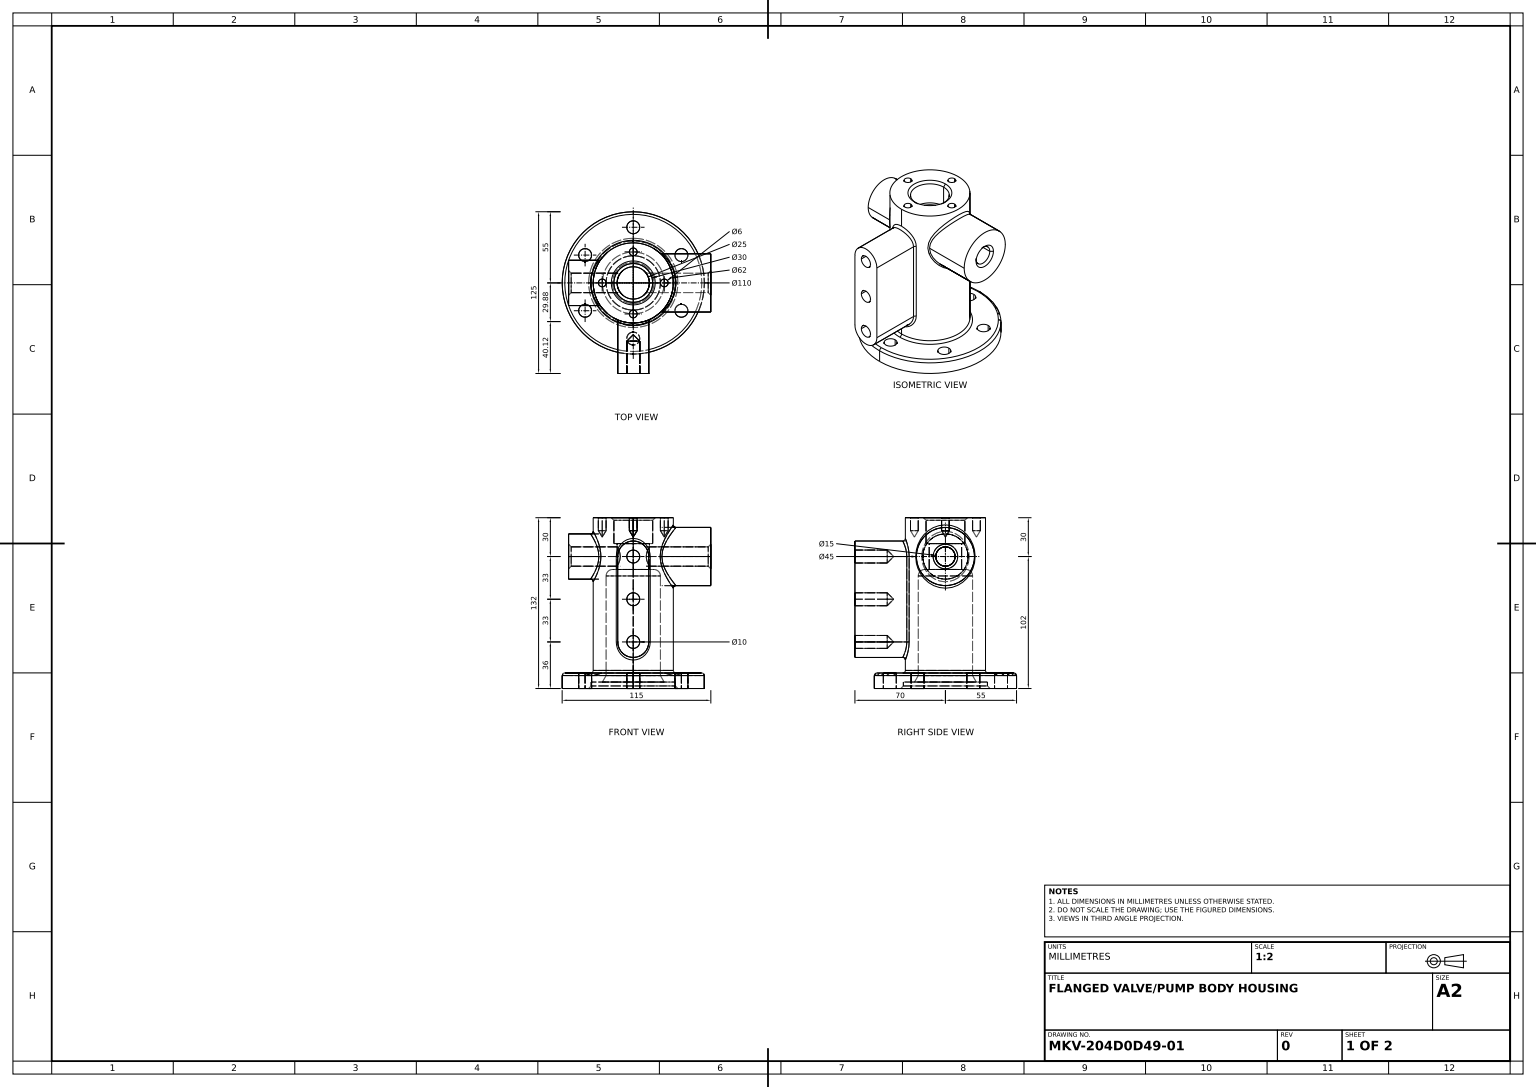
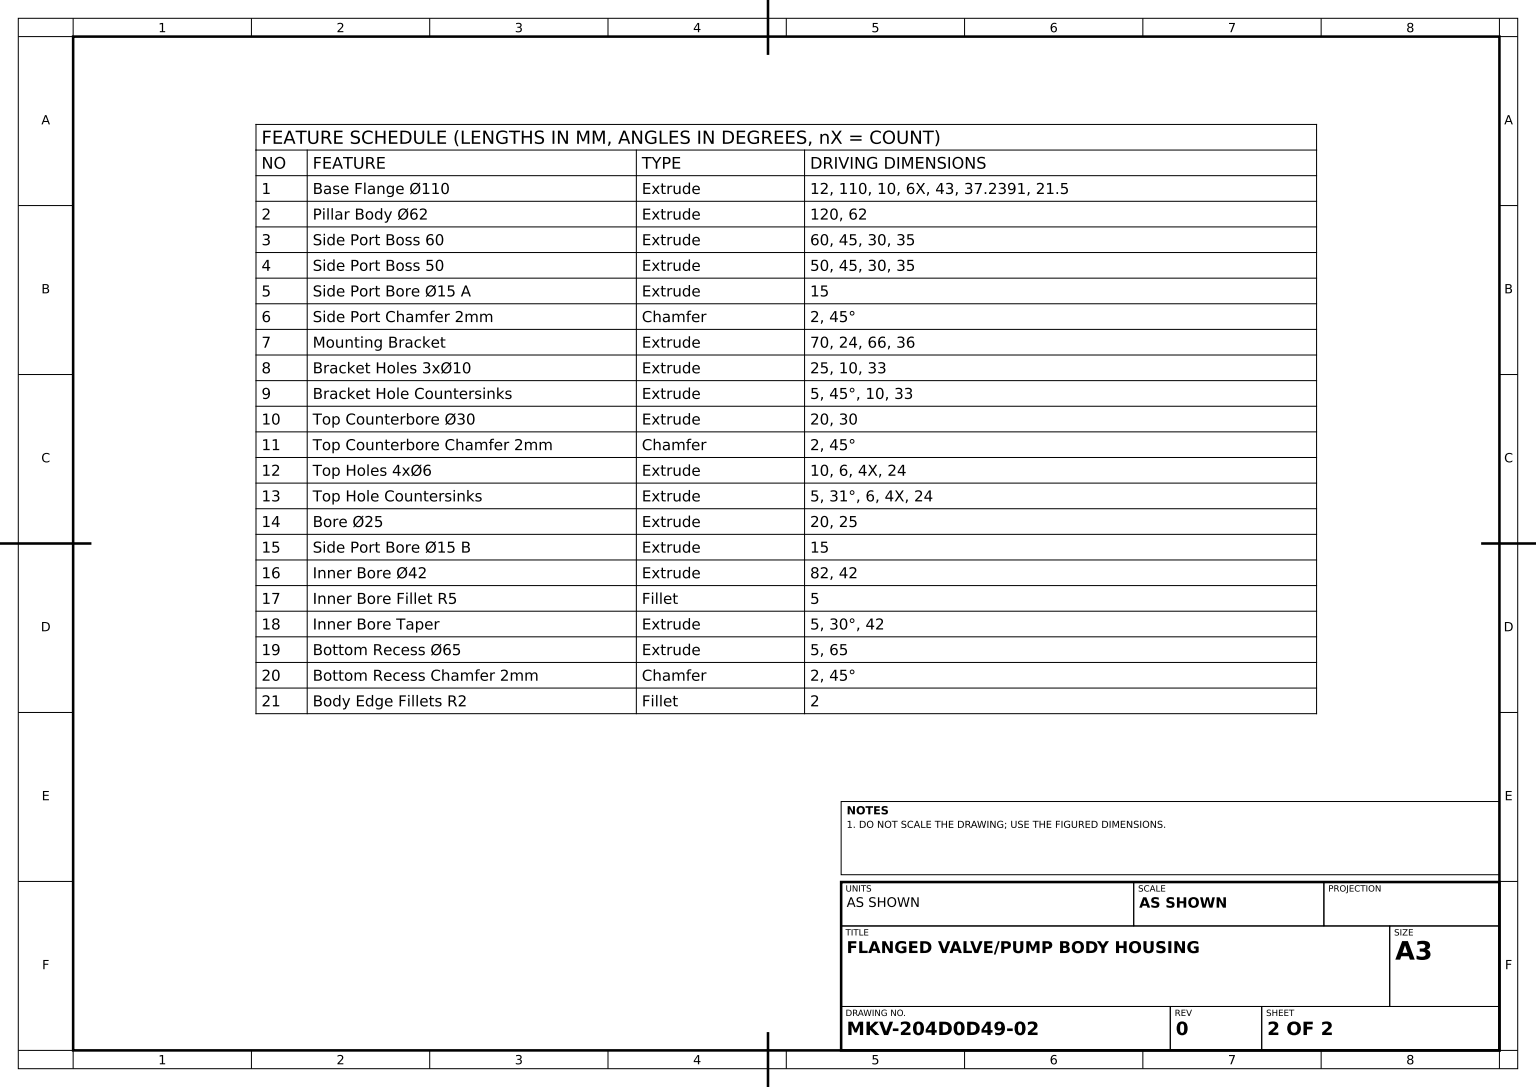
from build123d import *

# Parameters (mm, degrees)
BASE_FLANGE_SKETCH_R             = 55
BASE_FLANGE_SKETCH_R_2           = 5
BASE_FLANGE_110_DEPTH            = 12
PILLAR_BODY_SKETCH_R             = 31
PILLAR_BODY_62_DEPTH             = 120
SIDE_PORT_BOSSES_SKETCH_R        = 22.5
SIDE_PORT_BOSSES_SKETCH_R_2      = 17.5
SIDE_PORT_BOSS_60_DEPTH          = 60
SIDE_PORT_BOSS_50_DEPTH          = 50
SIDE_PORT_BORE_SKETCH_R          = 7.5
SIDE_PORT_BORE_15_A_DEPTH        = 184.504768402
SIDE_PORT_CHAMFER_2MM_SIZE       = 2
MOUNTING_BRACKET_DEPTH           = 70
BRACKET_HOLES_SKETCH_R           = 5
BRACKET_HOLES_3X_10_DEPTH        = 25
TOP_COUNTERBORE_SKETCH_R         = 15
TOP_COUNTERBORE_30_DEPTH         = 20
TOP_COUNTERBORE_CHAMFER_2MM_SIZE = 2
TOP_HOLES_SKETCH_R               = 3
TOP_HOLES_4X_6_DEPTH             = 10
BORE_25_SKETCH_R                 = 12.5
BORE_25_DEPTH                    = 20
SKETCH5_2_R                      = 7.5
SIDE_PORT_BORE_15_B_DEPTH        = 189.544424581
INNER_BORE_SKETCH_R              = 21
INNER_BORE_42_DEPTH              = 82
INNER_BORE_FILLET_R5_R           = 5
INNER_START                      = -82
SKETCH11_2_R                     = 21
INNER_BORE_TAPER_DEPTH           = 5
INNER_BORE_TAPER_DRAFT           = 30
BOTTOM_RECESS_SKETCH_R           = 32.5
BOTTOM_RECESS_65_DEPTH           = 5
BOTTOM_RECESS_CHAMFER_2MM_SIZE   = 2
BODY_EDGE_FILLETS_R2_R           = 2


with BuildPart() as part:
    # Base Flange Sketch → Base Flange _110 (new body)
    with BuildSketch(Plane(origin=(0, 0, 0), x_dir=(1, 0, 0), z_dir=(0, 1, 0))):
        with Locations(Location((0, 0, 0), (0, 0, 270))):
            Circle(BASE_FLANGE_SKETCH_R)
        with Locations(Location((0, 43, 0), (0, 0, 270))):
            Circle(BASE_FLANGE_SKETCH_R_2, mode=Mode.SUBTRACT)
        with Locations(Location((37.239092363, 21.5, 0), (0, 0, 270))):
            Circle(BASE_FLANGE_SKETCH_R_2, mode=Mode.SUBTRACT)
        with Locations(Location((37.239092363, -21.5, 0), (0, 0, 270))):
            Circle(BASE_FLANGE_SKETCH_R_2, mode=Mode.SUBTRACT)
        with Locations(Location((0, -43, 0), (0, 0, 270))):
            Circle(BASE_FLANGE_SKETCH_R_2, mode=Mode.SUBTRACT)
        with Locations(Location((-37.239092363, -21.5, 0), (0, 0, 270))):
            Circle(BASE_FLANGE_SKETCH_R_2, mode=Mode.SUBTRACT)
        with Locations(Location((-37.239092363, 21.5, 0), (0, 0, 270))):
            Circle(BASE_FLANGE_SKETCH_R_2, mode=Mode.SUBTRACT)
    extrude(amount=BASE_FLANGE_110_DEPTH)

    # Pillar Body Sketch → Pillar Body _62 (add)
    with BuildSketch(Plane(origin=(0, 12, 0), x_dir=(1, 0, 0), z_dir=(0, 1, 0))):
        with Locations(Location((0, 0, 0), (0, 0, 270))):
            Circle(PILLAR_BODY_SKETCH_R)
    extrude(amount=PILLAR_BODY_62_DEPTH)

    # Side Port Bosses Sketch → Side Port Boss 60 (add)
    # profile 1 of 5: a face of its own
    with BuildSketch(Plane(origin=(0, 0, 0), x_dir=(0, 0, -1), z_dir=(1, 0, 0))):
        with Locations(Location((0, 102, 0), (0, 0, 180))):
            Circle(SIDE_PORT_BOSSES_SKETCH_R)
        with Locations((0, 102)):
            Circle(SIDE_PORT_BOSSES_SKETCH_R_2, mode=Mode.SUBTRACT)
    # profile 2 of 5: a face of its own
    with BuildSketch(Plane(origin=(0, 0, 0), x_dir=(0, 0, -1), z_dir=(1, 0, 0))):
        with BuildLine():
            Line((17.5, 102), (-17.5, 102))
            ThreePointArc((-17.5, 102), (0, 84.5), (17.5, 102))
        make_face()
    # profile 3 of 5: a face of its own
    with BuildSketch(Plane(origin=(0, 0, 0), x_dir=(0, 0, -1), z_dir=(1, 0, 0))):
        with BuildLine():
            ThreePointArc((17.5, 102), (0, 119.5), (-17.5, 102))
            Line((-17.5, 102), (17.5, 102))
        make_face()
    # profile 4 of 5: a face of its own
    with BuildSketch(Plane(origin=(0, 0, 0), x_dir=(0, 0, -1), z_dir=(1, 0, 0))):
        with BuildLine():
            Line((17.5, 102), (-17.5, 102))
            ThreePointArc((-17.5, 102), (0, 84.5), (17.5, 102))
        make_face()
    # profile 5 of 5: a face of its own
    with BuildSketch(Plane(origin=(0, 0, 0), x_dir=(0, 0, -1), z_dir=(1, 0, 0))):
        with BuildLine():
            ThreePointArc((17.5, 102), (0, 119.5), (-17.5, 102))
            Line((-17.5, 102), (17.5, 102))
        make_face()
    extrude(amount=SIDE_PORT_BOSS_60_DEPTH)

    # Sketch4_3 → Side Port Boss 50 (add)
    with BuildSketch(Plane(origin=(0, 0, 0), x_dir=(0, 0, -1), z_dir=(1, 0, 0))):
        with BuildLine():
            ThreePointArc((17.5, 102), (0, 119.5), (-17.5, 102))
            Line((-17.5, 102), (17.5, 102))
        make_face()
        with BuildLine():
            Line((17.5, 102), (-17.5, 102))
            ThreePointArc((-17.5, 102), (0, 84.5), (17.5, 102))
        make_face()
        with BuildLine():
            ThreePointArc((17.5, 102), (0, 119.5), (-17.5, 102))
            Line((-17.5, 102), (17.5, 102))
        make_face()
        with BuildLine():
            Line((17.5, 102), (-17.5, 102))
            ThreePointArc((-17.5, 102), (0, 84.5), (17.5, 102))
        make_face()
    extrude(amount=-SIDE_PORT_BOSS_50_DEPTH)

    # Side Port Bore Sketch → Side Port Bore _15 A (cut, through all)
    with BuildSketch(Plane(origin=(60, 0, 0), x_dir=(0, 0, -1), z_dir=(1, 0, 0))):
        with Locations((0, 102)):
            Circle(SIDE_PORT_BORE_SKETCH_R)
    extrude(amount=-SIDE_PORT_BORE_15_A_DEPTH, mode=Mode.SUBTRACT)

    # Side Port Chamfer 2mm
    side_port_chamfer_2mm_edges = [part.edges().sort_by_distance(p)[0] for p in [
        (-50, 102, 7.5),
        (60, 102, 7.5),
    ]]
    chamfer(side_port_chamfer_2mm_edges, length=SIDE_PORT_CHAMFER_2MM_SIZE)

    # Mounting Bracket Sketch → Mounting Bracket (add)
    with BuildSketch(Plane.XY):
        with BuildLine():
            Line((-12, 36), (-12, 102))
            ThreePointArc((-12, 102), (0, 114), (12, 102))
            Line((12, 102), (12, 36))
            ThreePointArc((12, 36), (0, 24), (-12, 36))
        make_face()
    extrude(amount=MOUNTING_BRACKET_DEPTH)

    # Bracket Holes Sketch → Bracket Holes 3x_10 (cut)
    with BuildSketch(Plane.XY.offset(70)):
        with Locations((0, 102)):
            Circle(BRACKET_HOLES_SKETCH_R)
        with Locations((0, 69)):
            Circle(BRACKET_HOLES_SKETCH_R)
        with Locations((0, 36)):
            Circle(BRACKET_HOLES_SKETCH_R)
    extrude(amount=-BRACKET_HOLES_3X_10_DEPTH, mode=Mode.SUBTRACT)

    # Bracket Hole Countersinks cone 1 section (on through the dimple's axis) → Bracket Hole Countersinks (revolve, cut)
    with BuildSketch(Plane(origin=(0, 102, 45), x_dir=(0, -1, 0), z_dir=(1, 0, 0))):
        Polygon((0, 0), (5, 0), (0, 5), align=None)
    revolve(axis=Axis((0, 102, 45), (0, 0, -1)), mode=Mode.SUBTRACT)

    # Bracket Hole Countersinks cone 2 section (on through the dimple's axis) → Bracket Hole Countersinks cone 2 (revolve, cut)
    with BuildSketch(Plane(origin=(0, 69, 45), x_dir=(0, -1, 0), z_dir=(1, 0, 0))):
        Polygon((0, 0), (5, 0), (0, 5), align=None)
    revolve(axis=Axis((0, 69, 45), (0, 0, -1)), mode=Mode.SUBTRACT)

    # Bracket Hole Countersinks cone 3 section (on through the dimple's axis) → Bracket Hole Countersinks cone 3 (revolve, cut)
    with BuildSketch(Plane(origin=(0, 36, 45), x_dir=(0, -1, 0), z_dir=(1, 0, 0))):
        Polygon((0, 0), (5, 0), (0, 5), align=None)
    revolve(axis=Axis((0, 36, 45), (0, 0, -1)), mode=Mode.SUBTRACT)

    # Top Counterbore Sketch → Top Counterbore _30 (cut)
    with BuildSketch(Plane(origin=(0, 132, 0), x_dir=(1, 0, 0), z_dir=(0, 1, 0))):
        with Locations(Location((0, 0, 0), (0, 0, 270))):
            Circle(TOP_COUNTERBORE_SKETCH_R)
    extrude(amount=-TOP_COUNTERBORE_30_DEPTH, mode=Mode.SUBTRACT)

    # Top Counterbore Chamfer 2mm
    top_counterbore_chamfer_2mm_edges = [part.edges().sort_by_distance(p)[0] for p in [
        (0, 132, -15),
    ]]
    chamfer(top_counterbore_chamfer_2mm_edges, length=TOP_COUNTERBORE_CHAMFER_2MM_SIZE)

    # Top Holes Sketch → Top Holes 4x_6 (cut)
    with BuildSketch(Plane(origin=(0, 132, 0), x_dir=(1, 0, 0), z_dir=(0, 1, 0))):
        with Locations(Location((0, 24, 0), (0, 0, 270))):
            Circle(TOP_HOLES_SKETCH_R)
        with Locations(Location((24, 0, 0), (0, 0, 270))):
            Circle(TOP_HOLES_SKETCH_R)
        with Locations(Location((0, -24, 0), (0, 0, 270))):
            Circle(TOP_HOLES_SKETCH_R)
        with Locations(Location((-24, 0, 0), (0, 0, 270))):
            Circle(TOP_HOLES_SKETCH_R)
    extrude(amount=-TOP_HOLES_4X_6_DEPTH, mode=Mode.SUBTRACT)

    # Top Hole Countersinks cone 1 section (on through the dimple's axis) → Top Hole Countersinks (revolve, cut)
    with BuildSketch(Plane(origin=(0, 122, -24), x_dir=(0, 0, 1), z_dir=(1, 0, 0))):
        Polygon((0, 0), (3, 0), (0, 4.992838447), align=None)
    revolve(axis=Axis((0, 122, -24), (0, -1, 0)), mode=Mode.SUBTRACT)

    # Top Hole Countersinks cone 2 section (on through the dimple's axis) → Top Hole Countersinks cone 2 (revolve, cut)
    with BuildSketch(Plane(origin=(24, 122, 0), x_dir=(0, 0, 1), z_dir=(1, 0, 0))):
        Polygon((0, 0), (3, 0), (0, 4.992838447), align=None)
    revolve(axis=Axis((24, 122, 0), (0, -1, 0)), mode=Mode.SUBTRACT)

    # Top Hole Countersinks cone 3 section (on through the dimple's axis) → Top Hole Countersinks cone 3 (revolve, cut)
    with BuildSketch(Plane(origin=(0, 122, 24), x_dir=(0, 0, 1), z_dir=(1, 0, 0))):
        Polygon((0, 0), (3, 0), (0, 4.992838447), align=None)
    revolve(axis=Axis((0, 122, 24), (0, -1, 0)), mode=Mode.SUBTRACT)

    # Top Hole Countersinks cone 4 section (on through the dimple's axis) → Top Hole Countersinks cone 4 (revolve, cut)
    with BuildSketch(Plane(origin=(-24, 122, 0), x_dir=(0, 0, 1), z_dir=(1, 0, 0))):
        Polygon((0, 0), (3, 0), (0, 4.992838447), align=None)
    revolve(axis=Axis((-24, 122, 0), (0, -1, 0)), mode=Mode.SUBTRACT)

    # Bore _25 Sketch → Bore _25 (cut)
    with BuildSketch(Plane(origin=(0, 112, 0), x_dir=(1, 0, 0), z_dir=(0, 1, 0))):
        with Locations(Location((0, 0, 0), (0, 0, 270))):
            Circle(BORE_25_SKETCH_R)
    extrude(amount=-BORE_25_DEPTH, mode=Mode.SUBTRACT)

    # Sketch5_2 → Side Port Bore _15 B (cut, through all)
    with BuildSketch(Plane(origin=(60, 0, 0), x_dir=(0, 0, -1), z_dir=(1, 0, 0))):
        with Locations((0, 102)):
            Circle(SKETCH5_2_R)
    extrude(amount=-SIDE_PORT_BORE_15_B_DEPTH, mode=Mode.SUBTRACT)

    # Inner Bore Sketch → Inner Bore _42 (cut)
    with BuildSketch(Plane(origin=(0, 92, 0), x_dir=(1, 0, 0), z_dir=(0, 1, 0))):
        with Locations(Location((0, 0, 0), (0, 0, 270))):
            Circle(INNER_BORE_SKETCH_R)
    extrude(amount=-INNER_BORE_42_DEPTH, mode=Mode.SUBTRACT)

    # Inner Bore Fillet R5
    inner_bore_fillet_r5_edges = [part.edges().sort_by_distance(p)[0] for p in [
        (0, 92, -21),
    ]]
    fillet(inner_bore_fillet_r5_edges, radius=INNER_BORE_FILLET_R5_R)


with BuildPart() as inner_bore_taper_tool:
    # Sketch11_2 → Inner Bore Taper (with draft: the straight prism first)
    with BuildSketch(Plane(origin=(0, 92, 0), x_dir=(1, 0, 0), z_dir=(0, 1, 0)).offset(INNER_START)):
        with Locations(Location((0, 0, 0), (0, 0, 270))):
            Circle(SKETCH11_2_R)
    extrude(amount=-INNER_BORE_TAPER_DEPTH)
    # Inner Bore Taper: the draft: its side faces are tilted about the plane it starts from
    inner_bore_taper_sides = [inner_bore_taper_tool.faces().sort_by_distance(p)[0] for p in [
        (0, 7.5, -21),
    ]]
    draft(inner_bore_taper_sides, Plane(origin=(0, 92, 0), x_dir=(1, 0, 0), z_dir=(0, 1, 0)).offset(INNER_START), INNER_BORE_TAPER_DRAFT)


with BuildPart() as part_1:
    add(part.part)

    # Inner Bore Taper: cut by inner_bore_taper_tool
    add(inner_bore_taper_tool.part, mode=Mode.SUBTRACT)

    # Bottom Recess Sketch → Bottom Recess _65 (cut)
    with BuildSketch(Plane(origin=(0, 5, 0), x_dir=(1, 0, 0), z_dir=(0, 1, 0))):
        with Locations(Location((0, 0, 0), (0, 0, 270))):
            Circle(BOTTOM_RECESS_SKETCH_R)
    extrude(amount=-BOTTOM_RECESS_65_DEPTH, mode=Mode.SUBTRACT)

    # Bottom Recess Chamfer 2mm
    bottom_recess_chamfer_2mm_edges = [part_1.edges().sort_by_distance(p)[0] for p in [
        (0, 0, -32.5),
    ]]
    chamfer(bottom_recess_chamfer_2mm_edges, length=BOTTOM_RECESS_CHAMFER_2MM_SIZE)

    # Body Edge Fillets R2
    body_edge_fillets_r2_edges = [part_1.edges().sort_by_distance(p)[0] for p in [
        (0, 12, -31),
        (21.324868112, 102, -22.5),
        (-25.588083164, 102, 17.5),
        (0, 12, -55),
        (8.487533432, 27.516971282, 29.815462033),
        (0, 90.535533906, 19.535533906),
        (-12, 69, 28.583211856),
        (12, 69, 28.583211856),
    ]]
    fillet(body_edge_fillets_r2_edges, radius=BODY_EDGE_FILLETS_R2_R)


solid = part_1.part
